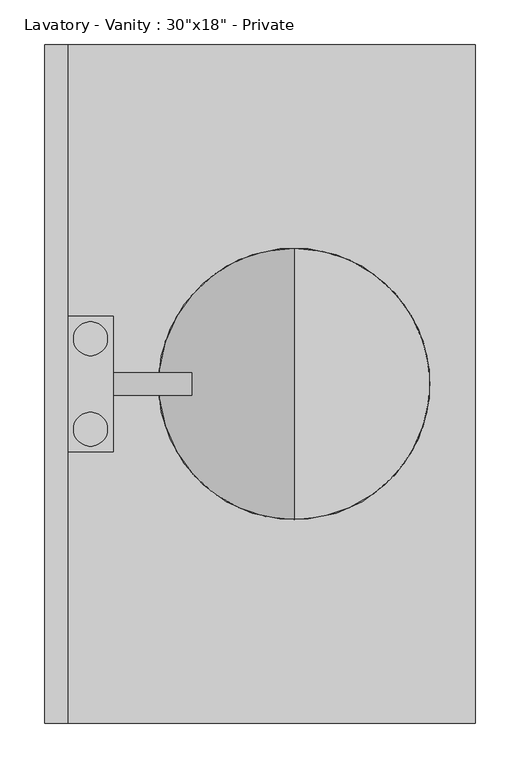
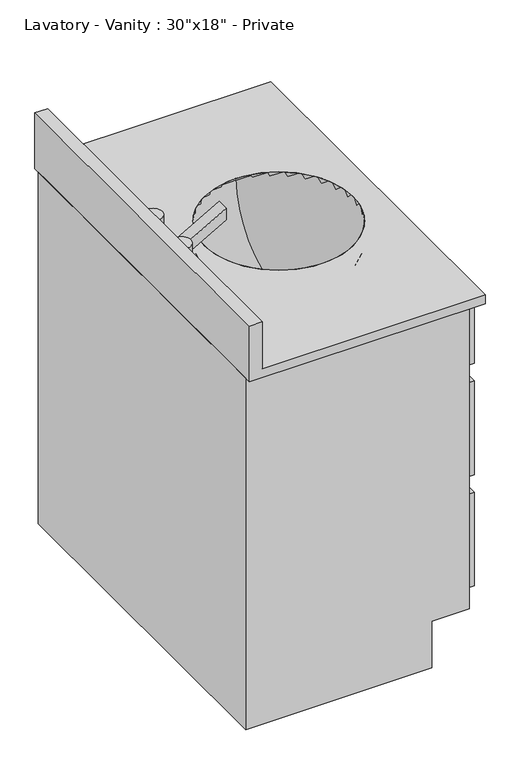
"""IFC4 building model written with IfcOpenShell, lengths in millimetres: flow terminal geometry."""

from ifc_helpers import new_model, si_unit, point, frame, origin, place, context, project, spatial, polyline, circle_curve, ellipse_curve, trimmed, faceted_brep, source, transform, mapped, element, save
from ifc_brep_helpers import plane_surface, cylinder_surface, revolved_surface, advanced_brep


def flow_terminal_15267b2a(model_context):
    return source(origin(), model_context, "Body", "SolidModel", [
        advanced_brep(
        [(32.54375, 50.8, 844.55), (70.64375, 50.8, 844.55), (32.54375, -50.8, 844.55), (70.64375, -50.8, 844.55), (32.54375, 50.8, 806.45), (70.64375, 50.8, 806.45), (32.54375, -50.8, 806.45), (70.64375, -50.8, 806.45), (76.99375, 76.2, 806.45), (26.19375, 76.2, 806.45), (26.19375, -76.2, 806.45), (76.99375, -76.2, 806.45), (76.99375, -12.7, 806.45), (76.99375, 12.7, 806.45), (76.99375, -76.2, 781.05), (26.19375, -76.2, 781.05), (26.19375, 76.2, 781.05), (76.99375, 76.2, 781.05), (76.99375, 12.7, 781.05), (76.99375, -12.7, 781.05), (165.1, -12.7, 831.85), (165.1, -12.7, 857.25), (165.1, 12.7, 857.25), (165.1, 12.7, 831.85)],
        [
            (0, 1, circle_curve(frame((51.59375, 50.8, 844.55), z_axis=(0.0, 0.0, 1.0), x_axis=(1.0, 0.0, 0.0)), 19.05)),
            (1, 0, circle_curve(frame((51.59375, 50.8, 844.55), z_axis=(0.0, 0.0, 1.0), x_axis=(1.0, 0.0, 0.0)), 19.05)),
            (2, 3, circle_curve(frame((51.59375, -50.8, 844.55), z_axis=(0.0, 0.0, 1.0), x_axis=(1.0, 0.0, 0.0)), 19.05)),
            (3, 2, circle_curve(frame((51.59375, -50.8, 844.55), z_axis=(0.0, 0.0, 1.0), x_axis=(1.0, 0.0, 0.0)), 19.05)),
            (0, 4),
            (4, 5, circle_curve(frame((51.59375, 50.8, 806.45), z_axis=(0.0, 0.0, 1.0), x_axis=(1.0, 0.0, 0.0)), 19.05)),
            (5, 1),
            (5, 4, circle_curve(frame((51.59375, 50.8, 806.45), z_axis=(0.0, 0.0, 1.0), x_axis=(1.0, 0.0, 0.0)), 19.05)),
            (2, 6),
            (6, 7, circle_curve(frame((51.59375, -50.8, 806.45), z_axis=(0.0, 0.0, 1.0), x_axis=(1.0, 0.0, 0.0)), 19.05)),
            (7, 3),
            (7, 6, circle_curve(frame((51.59375, -50.8, 806.45), z_axis=(0.0, 0.0, 1.0), x_axis=(1.0, 0.0, 0.0)), 19.05)),
            (8, 9),
            (9, 10),
            (10, 11),
            (11, 12),
            (12, 13),
            (13, 8),
            (14, 15),
            (15, 16),
            (16, 17),
            (17, 18),
            (18, 19),
            (19, 14),
            (8, 17),
            (16, 9),
            (15, 10),
            (14, 11),
            (13, 18),
            (19, 12),
            (19, 20),
            (20, 21),
            (21, 12),
            (13, 22),
            (22, 23),
            (23, 18),
            (23, 20),
            (22, 21),
        ],
        [
            plane_surface(frame((70.64375, 50.8, 844.55), z_axis=(0.0, 0.0, 1.0), x_axis=(0.0, 1.0, 0.0))),
            cylinder_surface(frame((51.59375, 50.8, 806.45), z_axis=(0.0, 0.0, 1.0), x_axis=(1.0, 0.0, 0.0)), 19.05),
            cylinder_surface(frame((51.59375, -50.8, 0.0), z_axis=(0.0, 0.0, 1.0), x_axis=(1.0, 0.0, 0.0)), 19.05),
            plane_surface(frame((26.19375, 76.2, 806.45), z_axis=(0.0, 0.0, 1.0), x_axis=(-1.0, 0.0, 0.0))),
            plane_surface(frame((26.19375, 76.2, 781.05), z_axis=(0.0, 0.0, -1.0), x_axis=(1.0, 0.0, 0.0))),
            plane_surface(frame((76.99375, 76.2, 806.45), z_axis=(0.0, 1.0, 0.0), x_axis=(0.0, 0.0, -1.0))),
            plane_surface(frame((26.19375, 76.2, 806.45), z_axis=(-1.0, 0.0, 0.0), x_axis=(0.0, 0.0, -1.0))),
            plane_surface(frame((26.19375, -76.2, 806.45), z_axis=(0.0, -1.0, 0.0), x_axis=(0.0, 0.0, -1.0))),
            plane_surface(frame((76.99375, -76.2, 806.45), z_axis=(1.0, 0.0, 0.0), x_axis=(0.0, 0.0, -1.0))),
            plane_surface(frame((76.99375, -12.7, 806.45), z_axis=(0.0, -1.0, 0.0), x_axis=(0.0, 0.0, -1.0))),
            plane_surface(frame((76.99375, 12.7, 806.45), z_axis=(0.0, 1.0, 0.0), x_axis=(0.0, 0.0, 1.0))),
            plane_surface(frame((76.99375, -12.7, 781.05), z_axis=(0.4994972193446417, 0.0, -0.8663154897997444), x_axis=(0.0, 1.0, 0.0))),
            plane_surface(frame((165.1, -12.7, 831.85), z_axis=(1.0, 0.0, 0.0), x_axis=(0.0, 1.0, 0.0))),
            plane_surface(frame((165.1, -12.7, 857.25), z_axis=(-0.4994972193446448, 0.0, 0.8663154897997426), x_axis=(0.0, 1.0, 0.0))),
        ],
        [
            (0, [[1, 2]]),
            (0, [[3, 4]]),
            (1, [[-1, 5, 6, 7]]),
            (1, [[-2, -7, 8, -5]]),
            (2, [[-3, 9, 10, 11]]),
            (2, [[-4, -11, 12, -9]]),
            (3, [[13, 14, 15, 16, 17, 18], [-6, -8], [-10, -12]]),
            (4, [[19, 20, 21, 22, 23, 24]]),
            (5, [[-13, 25, -21, 26]]),
            (6, [[-14, -26, -20, 27]]),
            (7, [[-15, -27, -19, 28]]),
            (8, [[-25, -18, 29, -22]]),
            (8, [[-28, -24, 30, -16]]),
            (9, [[31, 32, 33, -30]]),
            (10, [[34, 35, 36, -29]]),
            (11, [[-31, -23, -36, 37]]),
            (12, [[-32, -37, -35, 38]]),
            (13, [[-33, -38, -34, -17]]),
        ],
    ),
        faceted_brep([(381.79375, 368.3, 0.0), (381.79375, -368.3, 0.0), (0.0, -368.3, 0.0), (0.0, 368.3, 0.0), (0.0, 368.3, 762.0), (457.99375, 368.3, 762.0), (457.99375, 368.3, 101.6), (381.79375, 368.3, 101.6), (0.0, -368.3, 762.0), (381.79375, -368.3, 101.6), (457.99375, -368.3, 101.6), (457.99375, -368.3, 762.0), (26.19375, 342.9, 762.0), (445.29375, 342.9, 762.0), (445.29375, -342.9, 762.0), (26.19375, -342.9, 762.0), (457.99375, -342.9, 736.6), (457.99375, 342.9, 736.6), (457.99375, 342.9, 609.6), (457.99375, -342.9, 609.6), (457.99375, -342.9, 571.5), (457.99375, -88.9, 571.5), (457.99375, -88.9, 368.3), (457.99375, -342.9, 368.3), (457.99375, -342.9, 330.2), (457.99375, -88.9, 330.2), (457.99375, -88.9, 127.0), (457.99375, -342.9, 127.0), (457.99375, -50.8, 571.5), (457.99375, 342.9, 571.5), (457.99375, 342.9, 127.0), (457.99375, -50.8, 127.0), (445.29375, 342.9, 368.3), (26.19375, 342.9, 368.3), (26.19375, -342.9, 368.3), (445.29375, -342.9, 368.3), (483.39375, 342.9, 736.6), (483.39375, -342.9, 736.6), (483.39375, -342.9, 609.6), (483.39375, 342.9, 609.6), (483.39375, -88.9, 571.5), (483.39375, -342.9, 571.5), (483.39375, -342.9, 368.3), (483.39375, -88.9, 368.3), (483.39375, -88.9, 330.2), (483.39375, -342.9, 330.2), (483.39375, -342.9, 127.0), (483.39375, -88.9, 127.0), (483.39375, 342.9, 571.5), (483.39375, -50.8, 571.5), (483.39375, -50.8, 127.0), (483.39375, 342.9, 127.0)], [[[0, 1, 2, 3]], [[0, 3, 4, 5, 6, 7]], [[3, 2, 8, 4]], [[2, 1, 9, 10, 11, 8]], [[1, 0, 7, 9]], [[5, 4, 8, 11], [12, 13, 14, 15]], [[6, 10, 9, 7]], [[5, 11, 10, 6], [16, 17, 18, 19], [20, 21, 22, 23], [24, 25, 26, 27], [28, 29, 30, 31]], [[32, 33, 34, 35]], [[33, 32, 13, 12]], [[34, 33, 12, 15]], [[35, 34, 15, 14]], [[32, 35, 14, 13]], [[36, 37, 38, 39]], [[40, 41, 42, 43]], [[44, 45, 46, 47]], [[48, 49, 50, 51]], [[37, 36, 17, 16]], [[38, 37, 16, 19]], [[39, 38, 19, 18]], [[36, 39, 18, 17]], [[41, 40, 21, 20]], [[42, 41, 20, 23]], [[43, 42, 23, 22]], [[40, 43, 22, 21]], [[45, 44, 25, 24]], [[46, 45, 24, 27]], [[47, 46, 27, 26]], [[44, 47, 26, 25]], [[49, 48, 29, 28]], [[50, 49, 28, 31]], [[51, 50, 31, 30]], [[48, 51, 30, 29]]]),
        advanced_brep(
        [(483.39375, -381.0, 781.05), (483.39375, 381.0, 781.05), (26.19375, 381.0, 781.05), (26.19375, -381.0, 781.05), (432.59375, 0.0, 781.05), (127.79375, 0.0, 781.05), (483.39375, 381.0, 762.0), (483.39375, -381.0, 762.0), (0.0, -381.0, 762.0), (0.0, 381.0, 762.0), (127.79375, 0.0, 762.0), (432.59375, 0.0, 762.0), (0.0, 381.0, 882.65), (26.19375, 381.0, 882.65), (0.0, -381.0, 882.65), (26.19375, -381.0, 882.65)],
        [
            (0, 1),
            (1, 2),
            (2, 3),
            (3, 0),
            (4, 5, circle_curve(frame((280.19375, 0.0, 781.05), z_axis=(0.0, 0.0, -1.0), x_axis=(1.0, 0.0, 0.0)), 152.4)),
            (5, 4, circle_curve(frame((280.19375, 0.0, 781.05), z_axis=(0.0, 0.0, -1.0), x_axis=(1.0, 0.0, 0.0)), 152.4)),
            (6, 7),
            (7, 8),
            (8, 9),
            (9, 6),
            (10, 11, circle_curve(frame((280.19375, 0.0, 762.0), z_axis=(0.0, 0.0, 1.0), x_axis=(1.0, 0.0, 0.0)), 152.4)),
            (11, 10, circle_curve(frame((280.19375, 0.0, 762.0), z_axis=(0.0, 0.0, 1.0), x_axis=(1.0, 0.0, 0.0)), 152.4)),
            (9, 12),
            (12, 13),
            (13, 2),
            (1, 6),
            (8, 14),
            (14, 12),
            (7, 0),
            (3, 15),
            (15, 14),
            (4, 11),
            (10, 5),
            (15, 13),
        ],
        [
            plane_surface(frame((0.0, 381.0, 781.05), z_axis=(0.0, 0.0, 1.0), x_axis=(-1.0, 0.0, 0.0))),
            plane_surface(frame((0.0, 381.0, 762.0), z_axis=(0.0, 0.0, -1.0), x_axis=(1.0, 0.0, 0.0))),
            plane_surface(frame((483.39375, 381.0, 781.05), z_axis=(0.0, 1.0, 0.0), x_axis=(0.0, 0.0, -1.0))),
            plane_surface(frame((0.0, 381.0, 781.05), z_axis=(-1.0, 0.0, 0.0), x_axis=(0.0, 0.0, -1.0))),
            plane_surface(frame((0.0, -381.0, 781.05), z_axis=(0.0, -1.0, 0.0), x_axis=(0.0, 0.0, -1.0))),
            plane_surface(frame((483.39375, -381.0, 781.05), z_axis=(1.0, 0.0, 0.0), x_axis=(0.0, 0.0, -1.0))),
            revolved_surface(polyline([(432.59375, 0.0, 781.05), (432.59375, 0.0, 762.0)]), (280.19375, 0.0, 762.0), (0.0, 0.0, 1.0)),
            plane_surface(frame((0.0, 381.0, 882.65), z_axis=(0.0, 0.0, 1.0), x_axis=(-1.0, 0.0, 0.0))),
            plane_surface(frame((26.19375, -381.0, 882.65), z_axis=(1.0, 0.0, 0.0), x_axis=(0.0, 0.0, -1.0))),
        ],
        [
            (0, [[1, 2, 3, 4], [5, 6]]),
            (1, [[7, 8, 9, 10], [11, 12]]),
            (2, [[-10, 13, 14, 15, -2, 16]]),
            (3, [[-13, -9, 17, 18]]),
            (4, [[-17, -8, 19, -4, 20, 21]]),
            (5, [[-1, -19, -7, -16]]),
            (6, [[22, -11, 23, -5]]),
            (6, [[-22, -6, -23, -12]]),
            (7, [[-14, -18, -21, 24]]),
            (8, [[-24, -20, -3, -15]]),
        ],
    ),
        advanced_brep(
        [(280.19375, 0.0, 628.65), (280.19375, 152.4, 781.05), (280.19375, -152.4, 781.05), (280.19375, -44.45, 628.65), (280.19375, 44.45, 628.65), (280.19375, 0.0, 628.65), (280.19375, -157.6028553, 762.0), (280.19375, 157.6028553, 762.0)],
        [
            (0, 1, circle_curve(frame((280.19375, 0.0, 781.05), z_axis=(1.0, 0.0, 0.0), x_axis=(0.0, 1.0, 0.0)), 152.4)),
            (1, 2, circle_curve(frame((280.19375, 0.0, 781.05), z_axis=(0.0, 0.0, 1.0), x_axis=(0.0, 1.0, 0.0)), 152.4)),
            (2, 0, circle_curve(frame((280.19375, 0.0, 781.05), z_axis=(1.0, 0.0, 0.0), x_axis=(0.0, -1.0, 0.0)), 152.4)),
            (2, 1, circle_curve(frame((280.19375, 0.0, 781.05), z_axis=(0.0, 0.0, 1.0), x_axis=(0.0, 1.0, 0.0)), 152.4)),
            (3, 4, circle_curve(frame((280.19375, 0.0, 628.65), z_axis=(0.0, 0.0, -1.0), x_axis=(0.0, 1.0, 0.0)), 44.45)),
            (4, 5),
            (5, 3),
            (4, 3, circle_curve(frame((280.19375, 0.0, 628.65), z_axis=(0.0, 0.0, -1.0), x_axis=(0.0, 1.0, 0.0)), 44.45)),
            (6, 7, circle_curve(frame((280.19375, 0.0, 762.0), z_axis=(0.0, 0.0, -1.0), x_axis=(0.0, 1.0, 0.0)), 157.6028553)),
            (7, 4, circle_curve(frame((280.19375, 0.0, 781.05), z_axis=(-1.0, 0.0, 0.0), x_axis=(0.0, 1.0, 0.0)), 158.75)),
            (3, 6, circle_curve(frame((280.19375, 0.0, 781.05), z_axis=(-1.0, 0.0, 0.0), x_axis=(0.0, -1.0, 0.0)), 158.75)),
            (7, 6, circle_curve(frame((280.19375, 0.0, 762.0), z_axis=(0.0, 0.0, -1.0), x_axis=(0.0, 1.0, 0.0)), 157.6028553)),
            (1, 7),
            (6, 2),
        ],
        [
            revolved_surface(trimmed(ellipse_curve(frame((280.19375, 0.0, 781.05), z_axis=(-1.0, 0.0, 0.0), x_axis=(0.0, 1.0, 0.0)), 152.4, 152.4), [point((280.19375, 152.4, 781.05))], [point((280.19375, 0.0, 628.65))], True, "CARTESIAN"), (280.19375, 0.0, 520.7), (0.0, 0.0, 1.0)),
            plane_surface(frame((280.19375, 0.0, 628.65), z_axis=(0.0, 0.0, -1.0), x_axis=(0.0, 1.0, 0.0))),
            revolved_surface(trimmed(ellipse_curve(frame((280.19375, 0.0, 781.05), z_axis=(1.0, 0.0, 0.0), x_axis=(0.0, 1.0, 0.0)), 158.75, 158.75), [point((280.19375, 44.45, 628.65))], [point((280.19375, 157.6028553, 762.0))], True, "CARTESIAN"), (280.19375, 0.0, 520.7), (0.0, 0.0, 1.0)),
            revolved_surface(polyline([(280.19375, 157.6028553, 762.0), (280.19375, 152.4, 781.05)]), (280.19375, 0.0, 520.7), (0.0, 0.0, 1.0)),
        ],
        [
            (0, [[1, 2, 3]]),
            (0, [[-3, 4, -1]]),
            (1, [[5, 6, 7]]),
            (1, [[8, -7, -6]]),
            (2, [[9, 10, -5, 11]]),
            (2, [[12, -11, -8, -10]]),
            (3, [[-2, 13, -9, 14]]),
            (3, [[-4, -14, -12, -13]]),
        ],
    ),
    ])


if __name__ == "__main__":
    model = new_model("IFC4")
    model_context = context("Model", 3, world=origin())
    ifc_project = project(units=[si_unit("LENGTHUNIT", "METRE", prefix="MILLI")], contexts=[model_context])
    site = spatial("IfcSite", under=ifc_project)
    building = spatial("IfcBuilding", under=site)
    placement = place(None, origin())
    flow_terminal_shape = flow_terminal_15267b2a(model_context)
    element("IfcFlowTerminal", 1, ObjectType="Lavatory - Vanity : 30\"x18\" - Private", at=placement, inside=building, context=model_context, shape_type="MappedRepresentation", body=[
        mapped(flow_terminal_shape, transform((0.0, 0.0, 0.0), x_axis=(1.0, 0.0, 0.0), y_axis=(0.0, 1.0, 0.0), z_axis=(0.0, 0.0, 1.0))),
    ])
    save(model, "model.ifc")

# Revit data of these elements
# Type "Lavatory - Vanity : 30\"x18\" - Private"
#   Sanitary Radius = 5/8"
#   Sanitary Diameter = 1 1/4"
#   WFU = 1
#   Lavatory Length = 1' - 6"
#   Lavatory Width = 2' - 6"
#   Hot Water Radius = 1/4"
#   Hot Water Diameter = 1/2"
#   Half Lavatory Width = 1' - 3"
#   HWFU = 0.5
#   Flow Pressure [instance default] = 8.00 psi
#   Cold Water Radius = 1/4"
#   Cold Water Diameter = 1/2"
#   CWFU = 0.5
#   Sink Material = none
#   Faucet Material = none
#   Cabinet Top Material = none
#   Cabinet Material = none
#   Default Elevation = 0
